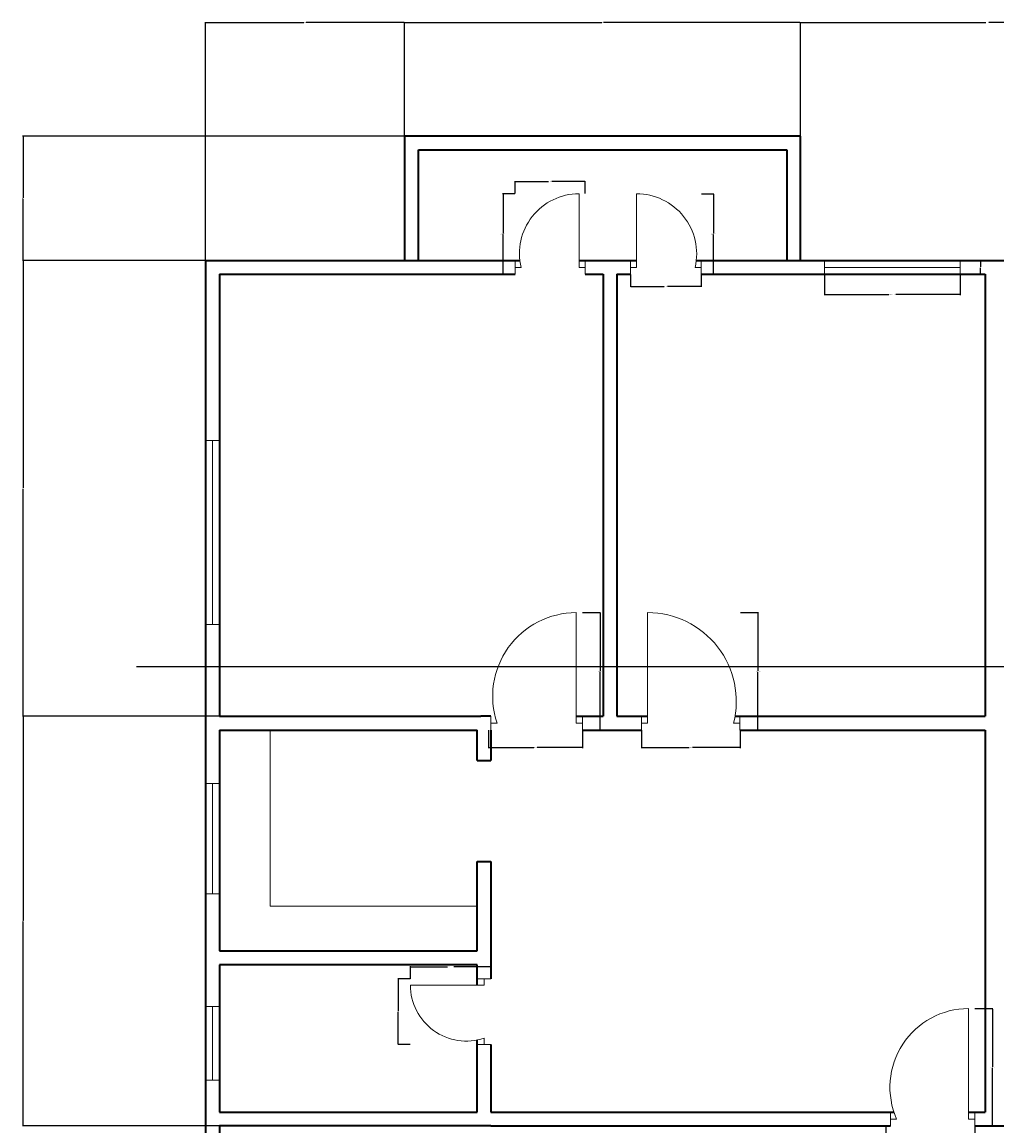
# Model space of a CAD drawing. Units: inches. Extents: x 1944 to 3454, y 1352 to 3055.
# Tile 13 of 17: x 2585 to 2903, y 1900 to 2260. Entities that reach past the tile are written whole.
import ezdxf

# ---------------------------------------------------------------- set-up
doc = ezdxf.new("R2010")
doc.units = ezdxf.units.IN
for name, color, linetype, lineweight in [('A-ANNO-DIMS', 2, 'Continuous', 18), ('A-ANNO-SYMB', 7, 'Continuous', 25), ('A-DOOR', 3, 'Continuous', 20), ('A-FLOR-CASE', 8, 'Continuous', 20), ('A-GLAZ', 4, 'Continuous', 18), ('A-WALL', 7, 'Continuous', 35)]:
    doc.layers.add(name, color=color, linetype=linetype, lineweight=lineweight)
doc.styles.get("Standard").update_dxf_attribs({"font": 'arial.ttf'})
doc.dimstyles.get("Standard").update_dxf_attribs({"dimtxt": 0.18, "dimasz": 0.18, "dimexe": 0.18, "dimexo": 0.0625, "dimgap": 0.09, "dimtad": 0, "dimtih": 1, "dimtoh": 1, "dimdec": 4, "dimzin": 0, "dimdsep": 46, "dimtxsty": 'Standard', "dimcen": 0.09, "dimadec": 0, "dimazin": 0, "dimtfac": 1, "dimtdec": 4, "dimtofl": 0, "dimtmove": 0, "dimatfit": 3, "dimfxl": 1, "dimtolj": 1, "dimtzin": 0, "dimarcsym": 0})

# ---------------------------------------------------------------- blocks, each defined once
blk = doc.blocks.new('DOOR-SWING-36IN-03')
for p, q in [((2, 2.25), (2, 38.25)), ((0, 4.5), (0, 0)), ((32, 4.5), (32, 0)), ((0, 0), (0, 2.25)), ((0, 2.25), (2, 2.25)), ((32, 2.25), (30, 2.25)), ((32, 0), (32, 2.25))]:
    blk.add_line(p, q)
blk.add_arc((2, 9.36), 28.89, 345.7565, 90)
blk = doc.blocks.new('DOOR-SWING-36IN-04')
for p, q in [((27.8, 2.25), (27.8, 38.25)), ((0, 0), (0, 4.5)), ((29.8, 4.5), (29.8, 0)), ((0, 2.25), (2, 2.25)), ((29.8, 2.25), (27.8, 2.25)), ((29.8, 0), (29.8, 2.25))]:
    blk.add_line(p, q)
blk.add_arc((27.8, 11), 27.25, 90, 198.7358)
blk = doc.blocks.new('DOOR-SWING-24IN-01')
for p, q in [((20.84, 2.25), (20.84, 26.25)), ((0, 4.5), (0, 0)), ((22.84, 0), (22.84, 4.5)), ((22.84, 4.5), (22.84, 2.25)), ((0, 0), (0, 2.25)), ((0, 2.25), (2, 2.25)), ((22.84, 2.25), (20.84, 2.25))]:
    blk.add_line(p, q)
blk.add_arc((20.84, 6.85), 19.4, 90, 193.7219)
blk = doc.blocks.new('DOOR-SWING-24IN-02')
for p, q in [((2, 2.25), (2, 26.25)), ((0, 0), (0, 4.5)), ((0, 4.5), (0, 2.25)), ((23.1, 4.5), (23.1, 0)), ((0, 2.25), (2, 2.25)), ((23.1, 2.25), (21.1, 2.25)), ((23.1, 0), (23.1, 2.25))]:
    blk.add_line(p, q)
blk.add_arc((2, 6.65), 19.6, 347.0256, 90)
blk = doc.blocks.new('DOOR-SWING-24IN-06')
for p, q in [((24, 19.31), (0, 19.31)), ((21.75, 21.31), (26.25, 21.31)), ((26.25, 21.31), (24, 21.31)), ((24, 21.31), (24, 19.31)), ((24, 0), (24, 2)), ((21.75, 0), (26.25, 0)), ((26.25, 0), (24, 0))]:
    blk.add_line(p, q)
blk.add_arc((18.24, 19.31), 18.24, 180, 288.4122)
blk = doc.blocks.new('DOOR-SWING-36IN-10')
for p, q in [((25.63, 2.25), (25.63, 38.25)), ((0.18, 4.5), (0.18, 0)), ((27.63, 4.5), (27.63, 0)), ((0.18, 0), (0.18, 2.25)), ((0.18, 2.25), (2.18, 2.25)), ((27.63, 2.25), (25.63, 2.25)), ((27.63, 0), (27.63, 2.25))]:
    blk.add_line(p, q)
blk.add_arc((25.63, 12.61), 25.64, 90, 203.8432)
blk = doc.blocks.new('WINDOW-PLAN-60.00IN-01')
for p, q in [((0, 60), (4.5, 60)), ((4.5, 60), (2.25, 60)), ((2.25, 60), (2.25, 0)), ((4.5, 0), (0, 0)), ((2.25, 0), (4.5, 0))]:
    blk.add_line(p, q)
blk = doc.blocks.new('WINDOW-PLAN-36.00IN-01')
for p, q in [((0, 36), (4.5, 36)), ((4.5, 36), (2.25, 36)), ((2.25, 36), (2.25, 0)), ((2.25, 0), (0, 0)), ((0, 0), (4.5, 0))]:
    blk.add_line(p, q)
blk = doc.blocks.new('WINDOW-PLAN-24.00IN-01')
for p, q in [((2.25, 24), (0, 24)), ((0, 24), (4.5, 24)), ((2.25, 0), (2.25, 24)), ((0, 0), (4.5, 0)), ((4.5, 0), (2.25, 0))]:
    blk.add_line(p, q)
blk = doc.blocks.new('WINDOW-PLAN-44.19IN-01')
for p, q in [((0, 4.5), (0, 0)), ((44.19, 2.25), (44.19, 4.5)), ((44.19, 4.5), (44.19, 0)), ((0, 0), (0, 2.25)), ((0, 2.25), (44.19, 2.25))]:
    blk.add_line(p, q)
blk = doc.blocks.new('*D86')
at = {"layer": 'A-ANNO-DIMS', "color": 0, "lineweight": -2, "transparency": 16777216}
for p, q in [((2846.55, 2177.53), (2846.55, 2170.79)), ((2890.74, 2177.53), (2890.74, 2170.79)), ((2846.73, 2170.97), (2867.52, 2170.97)), ((2890.56, 2170.97), (2869.76, 2170.97))]:
    blk.add_line(p, q, dxfattribs=at)
at = {"layer": 'A-ANNO-DIMS', "color": 0, "transparency": 16777216}
for points in [[(2846.73, 2171), (2846.73, 2170.94), (2846.55, 2170.97)], [(2890.56, 2171), (2890.56, 2170.94), (2890.74, 2170.97)]]:
    blk.add_solid(points, dxfattribs=at)
at = {"layer": 'Defpoints', "color": 0, "transparency": 16777216}
for p in [(2846.55, 2177.6), (2890.74, 2177.6), (2890.74, 2170.97)]:
    blk.add_point(p, dxfattribs=at)
at = {"layer": 'A-ANNO-DIMS', "color": 0, "transparency": 16777216, "insert": (2868.64, 2170.97), "char_height": 0.18, "attachment_point": 5}
blk.add_mtext('\\A1;WINDOW 44 TYP.', dxfattribs=at)
blk = doc.blocks.new('*D87')
at = {"layer": 'A-ANNO-DIMS', "color": 0, "lineweight": -2, "transparency": 16777216}
for p, q in [((2890.8, 2182.1), (2897.55, 2182.1)), ((2897.37, 2181.92), (2897.37, 2180.03)), ((2897.37, 2177.78), (2897.37, 2179.66)), ((2890.8, 2177.6), (2897.55, 2177.6))]:
    blk.add_line(p, q, dxfattribs=at)
at = {"layer": 'A-ANNO-DIMS', "color": 0, "transparency": 16777216}
for points in [[(2897.34, 2181.92), (2897.4, 2181.92), (2897.37, 2182.1)], [(2897.34, 2177.78), (2897.4, 2177.78), (2897.37, 2177.6)]]:
    blk.add_solid(points, dxfattribs=at)
at = {"layer": 'Defpoints', "color": 0, "transparency": 16777216}
for p in [(2890.74, 2182.1), (2897.37, 2182.1), (2890.74, 2177.6)]:
    blk.add_point(p, dxfattribs=at)
at = {"layer": 'A-ANNO-DIMS', "color": 0, "transparency": 16777216, "insert": (2897.37, 2179.85), "char_height": 0.18, "attachment_point": 5}
blk.add_mtext('\\A1;5 TYP.', dxfattribs=at)
blk = doc.blocks.new('*D96')
at = {"layer": 'A-ANNO-DIMS', "color": 0, "lineweight": -2, "transparency": 16777216}
for p, q in [((2819.16, 2067.35), (2825.02, 2067.35)), ((2824.84, 2067.17), (2824.84, 2048.4)), ((2824.84, 2029.28), (2824.84, 2048.04)), ((2819.16, 2029.1), (2825.02, 2029.1))]:
    blk.add_line(p, q, dxfattribs=at)
at = {"layer": 'A-ANNO-DIMS', "color": 0, "transparency": 16777216}
for points in [[(2824.81, 2067.17), (2824.87, 2067.17), (2824.84, 2067.35)], [(2824.81, 2029.28), (2824.87, 2029.28), (2824.84, 2029.1)]]:
    blk.add_solid(points, dxfattribs=at)
at = {"layer": 'Defpoints', "color": 0, "transparency": 16777216}
for p in [(2819.1, 2067.35), (2824.84, 2067.35), (2819.1, 2029.1)]:
    blk.add_point(p, dxfattribs=at)
at = {"layer": 'A-ANNO-DIMS', "color": 0, "transparency": 16777216, "insert": (2824.84, 2048.22), "char_height": 0.18, "attachment_point": 5}
blk.add_mtext('\\A1;SWING 38 TYP.', dxfattribs=at)
blk = doc.blocks.new('*D97')
at = {"layer": 'A-ANNO-DIMS', "color": 0, "lineweight": -2, "transparency": 16777216}
for p, q in [((2786.9, 2029.03), (2786.9, 2023.18)), ((2819.1, 2029.03), (2819.1, 2023.18)), ((2787.08, 2023.36), (2802.48, 2023.36)), ((2818.92, 2023.36), (2803.53, 2023.36))]:
    blk.add_line(p, q, dxfattribs=at)
at = {"layer": 'A-ANNO-DIMS', "color": 0, "transparency": 16777216}
for points in [[(2787.08, 2023.39), (2787.08, 2023.33), (2786.9, 2023.36)], [(2818.92, 2023.39), (2818.92, 2023.33), (2819.1, 2023.36)]]:
    blk.add_solid(points, dxfattribs=at)
at = {"layer": 'Defpoints', "color": 0, "transparency": 16777216}
for p in [(2786.9, 2029.1), (2819.1, 2029.1), (2819.1, 2023.36)]:
    blk.add_point(p, dxfattribs=at)
at = {"layer": 'A-ANNO-DIMS', "color": 0, "transparency": 16777216, "insert": (2803, 2023.36), "char_height": 0.18, "attachment_point": 5}
blk.add_mtext('\\A1;32 TYP.', dxfattribs=at)
blk = doc.blocks.new('*D98')
at = {"layer": 'A-ANNO-DIMS', "color": 0, "lineweight": -2, "transparency": 16777216}
for p, q in [((2767.74, 2067.35), (2773.6, 2067.35)), ((2773.42, 2067.17), (2773.42, 2048.4)), ((2773.42, 2029.28), (2773.42, 2048.04)), ((2767.74, 2029.1), (2773.6, 2029.1))]:
    blk.add_line(p, q, dxfattribs=at)
at = {"layer": 'A-ANNO-DIMS', "color": 0, "transparency": 16777216}
for points in [[(2773.39, 2067.17), (2773.45, 2067.17), (2773.42, 2067.35)], [(2773.39, 2029.28), (2773.45, 2029.28), (2773.42, 2029.1)]]:
    blk.add_solid(points, dxfattribs=at)
at = {"layer": 'Defpoints', "color": 0, "transparency": 16777216}
for p in [(2767.68, 2067.35), (2773.42, 2067.35), (2767.68, 2029.1)]:
    blk.add_point(p, dxfattribs=at)
at = {"layer": 'A-ANNO-DIMS', "color": 0, "transparency": 16777216, "insert": (2773.42, 2048.22), "char_height": 0.18, "attachment_point": 5}
blk.add_mtext('\\A1;SWING 38 TYP.', dxfattribs=at)
blk = doc.blocks.new('*D99')
at = {"layer": 'A-ANNO-DIMS', "color": 0, "lineweight": -2, "transparency": 16777216}
for p, q in [((2737.05, 2029.03), (2737.05, 2023.18)), ((2767.68, 2029.03), (2767.68, 2023.18)), ((2737.23, 2023.36), (2751.84, 2023.36)), ((2767.5, 2023.36), (2752.89, 2023.36))]:
    blk.add_line(p, q, dxfattribs=at)
at = {"layer": 'A-ANNO-DIMS', "color": 0, "transparency": 16777216}
for points in [[(2737.23, 2023.39), (2737.23, 2023.33), (2737.05, 2023.36)], [(2767.5, 2023.39), (2767.5, 2023.33), (2767.68, 2023.36)]]:
    blk.add_solid(points, dxfattribs=at)
at = {"layer": 'Defpoints', "color": 0, "transparency": 16777216}
for p in [(2737.05, 2029.1), (2767.68, 2029.1), (2767.68, 2023.36)]:
    blk.add_point(p, dxfattribs=at)
at = {"layer": 'A-ANNO-DIMS', "color": 0, "transparency": 16777216, "insert": (2752.37, 2023.36), "char_height": 0.18, "attachment_point": 5}
blk.add_mtext('\\A1;31 TYP.', dxfattribs=at)
blk = doc.blocks.new('*D110')
at = {"layer": 'A-ANNO-DIMS', "color": 0, "lineweight": -2, "transparency": 16777216}
for p, q in [((2895.56, 1938.35), (2901.41, 1938.35)), ((2901.23, 1938.17), (2901.23, 1919.4)), ((2901.23, 1900.28), (2901.23, 1919.04)), ((2895.56, 1900.1), (2901.41, 1900.1))]:
    blk.add_line(p, q, dxfattribs=at)
at = {"layer": 'A-ANNO-DIMS', "color": 0, "transparency": 16777216}
for points in [[(2901.2, 1938.17), (2901.26, 1938.17), (2901.23, 1938.35)], [(2901.2, 1900.28), (2901.26, 1900.28), (2901.23, 1900.1)]]:
    blk.add_solid(points, dxfattribs=at)
at = {"layer": 'Defpoints', "color": 0, "transparency": 16777216}
for p in [(2895.49, 1938.35), (2901.23, 1938.35), (2895.49, 1900.1)]:
    blk.add_point(p, dxfattribs=at)
at = {"layer": 'A-ANNO-DIMS', "color": 0, "transparency": 16777216, "insert": (2901.23, 1919.22), "char_height": 0.18, "attachment_point": 5}
blk.add_mtext('\\A1;SWING 38 TYP.', dxfattribs=at)
blk = doc.blocks.new('*D111')
at = {"layer": 'A-ANNO-DIMS', "color": 0, "lineweight": -2, "transparency": 16777216}
for p, q in [((2866.54, 1900.03), (2866.54, 1894.18)), ((2895.49, 1900.03), (2895.49, 1894.18)), ((2866.72, 1894.36), (2880.49, 1894.36)), ((2895.31, 1894.36), (2881.55, 1894.36))]:
    blk.add_line(p, q, dxfattribs=at)
at = {"layer": 'A-ANNO-DIMS', "color": 0, "transparency": 16777216}
for points in [[(2866.72, 1894.39), (2866.72, 1894.33), (2866.54, 1894.36)], [(2895.31, 1894.39), (2895.31, 1894.33), (2895.49, 1894.36)]]:
    blk.add_solid(points, dxfattribs=at)
at = {"layer": 'Defpoints', "color": 0, "transparency": 16777216}
for p in [(2866.54, 1900.1), (2895.49, 1900.1), (2895.49, 1894.36)]:
    blk.add_point(p, dxfattribs=at)
at = {"layer": 'A-ANNO-DIMS', "color": 0, "transparency": 16777216, "insert": (2881.02, 1894.36), "char_height": 0.18, "attachment_point": 5}
blk.add_mtext('\\A1;29 TYP.', dxfattribs=at)
blk = doc.blocks.new('*D116')
at = {"layer": 'A-ANNO-DIMS', "color": 0, "lineweight": -2, "transparency": 16777216}
for p, q in [((2745.67, 2203.85), (2741.62, 2203.85)), ((2741.8, 2203.67), (2741.8, 2190.9)), ((2741.8, 2177.78), (2741.8, 2190.54)), ((2745.67, 2177.6), (2741.62, 2177.6))]:
    blk.add_line(p, q, dxfattribs=at)
at = {"layer": 'A-ANNO-DIMS', "color": 0, "transparency": 16777216}
for points in [[(2741.77, 2203.67), (2741.83, 2203.67), (2741.8, 2203.85)], [(2741.77, 2177.78), (2741.83, 2177.78), (2741.8, 2177.6)]]:
    blk.add_solid(points, dxfattribs=at)
at = {"layer": 'Defpoints', "color": 0, "transparency": 16777216}
for p in [(2741.8, 2203.85), (2745.73, 2203.85), (2745.73, 2177.6)]:
    blk.add_point(p, dxfattribs=at)
at = {"layer": 'A-ANNO-DIMS', "color": 0, "transparency": 16777216, "insert": (2741.8, 2190.72), "char_height": 0.18, "attachment_point": 5}
blk.add_mtext('\\A1;SWING 26 TYP.', dxfattribs=at)
blk = doc.blocks.new('*D117')
at = {"layer": 'A-ANNO-DIMS', "color": 0, "lineweight": -2, "transparency": 16777216}
for p, q in [((2745.73, 2203.91), (2745.73, 2207.96)), ((2745.91, 2207.78), (2756.63, 2207.78)), ((2768.4, 2207.78), (2757.69, 2207.78)), ((2768.58, 2203.91), (2768.58, 2207.96))]:
    blk.add_line(p, q, dxfattribs=at)
at = {"layer": 'A-ANNO-DIMS', "color": 0, "transparency": 16777216}
for points in [[(2745.91, 2207.81), (2745.91, 2207.75), (2745.73, 2207.78)], [(2768.4, 2207.81), (2768.4, 2207.75), (2768.58, 2207.78)]]:
    blk.add_solid(points, dxfattribs=at)
at = {"layer": 'Defpoints', "color": 0, "transparency": 16777216}
for p in [(2768.58, 2207.78), (2745.73, 2203.85), (2768.58, 2203.85)]:
    blk.add_point(p, dxfattribs=at)
at = {"layer": 'A-ANNO-DIMS', "color": 0, "transparency": 16777216, "insert": (2757.16, 2207.78), "char_height": 0.18, "attachment_point": 5}
blk.add_mtext('\\A1;23 TYP.', dxfattribs=at)
blk = doc.blocks.new('*D118')
at = {"layer": 'A-ANNO-DIMS', "color": 0, "lineweight": -2, "transparency": 16777216}
for p, q in [((2806.45, 2203.85), (2810.51, 2203.85)), ((2810.33, 2203.67), (2810.33, 2190.9)), ((2810.33, 2177.78), (2810.33, 2190.54)), ((2806.45, 2177.6), (2810.51, 2177.6))]:
    blk.add_line(p, q, dxfattribs=at)
at = {"layer": 'A-ANNO-DIMS', "color": 0, "transparency": 16777216}
for points in [[(2810.3, 2203.67), (2810.36, 2203.67), (2810.33, 2203.85)], [(2810.3, 2177.78), (2810.36, 2177.78), (2810.33, 2177.6)]]:
    blk.add_solid(points, dxfattribs=at)
at = {"layer": 'Defpoints', "color": 0, "transparency": 16777216}
for p in [(2806.39, 2203.85), (2810.33, 2203.85), (2806.39, 2177.6)]:
    blk.add_point(p, dxfattribs=at)
at = {"layer": 'A-ANNO-DIMS', "color": 0, "transparency": 16777216, "insert": (2810.33, 2190.72), "char_height": 0.18, "attachment_point": 5}
blk.add_mtext('\\A1;SWING 26 TYP.', dxfattribs=at)
blk = doc.blocks.new('*D119')
at = {"layer": 'A-ANNO-DIMS', "color": 0, "lineweight": -2, "transparency": 16777216}
for p, q in [((2783.29, 2177.53), (2783.29, 2173.48)), ((2806.39, 2177.53), (2806.39, 2173.48)), ((2783.47, 2173.66), (2794.31, 2173.66)), ((2806.21, 2173.66), (2795.37, 2173.66))]:
    blk.add_line(p, q, dxfattribs=at)
at = {"layer": 'A-ANNO-DIMS', "color": 0, "transparency": 16777216}
for points in [[(2783.47, 2173.69), (2783.47, 2173.63), (2783.29, 2173.66)], [(2806.21, 2173.69), (2806.21, 2173.63), (2806.39, 2173.66)]]:
    blk.add_solid(points, dxfattribs=at)
at = {"layer": 'Defpoints', "color": 0, "transparency": 16777216}
for p in [(2783.29, 2177.6), (2806.39, 2177.6), (2806.39, 2173.66)]:
    blk.add_point(p, dxfattribs=at)
at = {"layer": 'A-ANNO-DIMS', "color": 0, "transparency": 16777216, "insert": (2794.84, 2173.66), "char_height": 0.18, "attachment_point": 5}
blk.add_mtext('\\A1;23 TYP.', dxfattribs=at)
blk = doc.blocks.new('*D126')
at = {"layer": 'A-ANNO-DIMS', "color": 0, "lineweight": -2, "transparency": 16777216}
for p, q in [((2711.63, 1948.05), (2711.63, 1952.1)), ((2711.81, 1951.92), (2723.76, 1951.92)), ((2737.7, 1951.92), (2725.74, 1951.92)), ((2737.88, 1948.05), (2737.88, 1952.1))]:
    blk.add_line(p, q, dxfattribs=at)
at = {"layer": 'A-ANNO-DIMS', "color": 0, "transparency": 16777216}
for points in [[(2711.81, 1951.95), (2711.81, 1951.89), (2711.63, 1951.92)], [(2737.7, 1951.95), (2737.7, 1951.89), (2737.88, 1951.92)]]:
    blk.add_solid(points, dxfattribs=at)
at = {"layer": 'Defpoints', "color": 0, "transparency": 16777216}
for p in [(2737.88, 1951.92), (2711.63, 1947.99), (2737.88, 1947.99)]:
    blk.add_point(p, dxfattribs=at)
at = {"layer": 'A-ANNO-DIMS', "color": 0, "transparency": 16777216, "insert": (2724.75, 1951.92), "char_height": 0.18, "attachment_point": 5}
blk.add_mtext('\\A1;SWING 26 TYP.', dxfattribs=at)
blk = doc.blocks.new('*D127')
at = {"layer": 'A-ANNO-DIMS', "color": 0, "lineweight": -2, "transparency": 16777216}
for p, q in [((2711.56, 1947.99), (2707.51, 1947.99)), ((2707.69, 1947.81), (2707.69, 1937.51)), ((2707.69, 1926.86), (2707.69, 1937.15)), ((2711.56, 1926.68), (2707.51, 1926.68))]:
    blk.add_line(p, q, dxfattribs=at)
at = {"layer": 'A-ANNO-DIMS', "color": 0, "transparency": 16777216}
for points in [[(2707.66, 1947.81), (2707.72, 1947.81), (2707.69, 1947.99)], [(2707.66, 1926.86), (2707.72, 1926.86), (2707.69, 1926.68)]]:
    blk.add_solid(points, dxfattribs=at)
at = {"layer": 'Defpoints', "color": 0, "transparency": 16777216}
for p in [(2707.69, 1947.99), (2711.63, 1947.99), (2711.63, 1926.68)]:
    blk.add_point(p, dxfattribs=at)
at = {"layer": 'A-ANNO-DIMS', "color": 0, "transparency": 16777216, "insert": (2707.69, 1937.33), "char_height": 0.18, "attachment_point": 5}
blk.add_mtext('\\A1;21 TYP.', dxfattribs=at)
blk = doc.blocks.new('*D188')
at = {"layer": 'A-ANNO-DIMS', "color": 0, "lineweight": -2, "transparency": 16777216}
for p, q in [((2644.81, 2182.1), (2585.24, 2182.1)), ((2585.42, 2181.92), (2585.42, 2108.03)), ((2585.42, 2033.78), (2585.42, 2107.66)), ((2649.31, 2033.6), (2585.24, 2033.6))]:
    blk.add_line(p, q, dxfattribs=at)
at = {"layer": 'A-ANNO-DIMS', "color": 0, "transparency": 16777216}
for points in [[(2585.39, 2181.92), (2585.45, 2181.92), (2585.42, 2182.1)], [(2585.39, 2033.78), (2585.45, 2033.78), (2585.42, 2033.6)]]:
    blk.add_solid(points, dxfattribs=at)
at = {"layer": 'Defpoints', "color": 0, "transparency": 16777216}
for p in [(2644.88, 2182.1), (2585.42, 2033.6), (2649.38, 2033.6)]:
    blk.add_point(p, dxfattribs=at)
at = {"layer": 'A-ANNO-DIMS', "color": 0, "transparency": 16777216, "insert": (2585.42, 2107.85), "char_height": 0.18, "attachment_point": 5}
blk.add_mtext('\\A1;148.5', dxfattribs=at)
blk = doc.blocks.new('*D189')
at = {"layer": 'A-ANNO-DIMS', "color": 0, "lineweight": -2, "transparency": 16777216}
for p, q in [((2649.31, 2033.6), (2585.24, 2033.6)), ((2585.42, 2033.42), (2585.42, 1967.03)), ((2585.42, 1900.28), (2585.42, 1966.66)), ((2649.31, 1900.1), (2585.24, 1900.1))]:
    blk.add_line(p, q, dxfattribs=at)
at = {"layer": 'A-ANNO-DIMS', "color": 0, "transparency": 16777216}
for points in [[(2585.39, 2033.42), (2585.45, 2033.42), (2585.42, 2033.6)], [(2585.39, 1900.28), (2585.45, 1900.28), (2585.42, 1900.1)]]:
    blk.add_solid(points, dxfattribs=at)
at = {"layer": 'Defpoints', "color": 0, "transparency": 16777216}
for p in [(2649.38, 2033.6), (2585.42, 1900.1), (2649.38, 1900.1)]:
    blk.add_point(p, dxfattribs=at)
at = {"layer": 'A-ANNO-DIMS', "color": 0, "transparency": 16777216, "insert": (2585.42, 1966.85), "char_height": 0.18, "attachment_point": 5}
blk.add_mtext('\\A1;133.5', dxfattribs=at)
blk = doc.blocks.new('*D193')
at = {"layer": 'A-ANNO-DIMS', "color": 0, "lineweight": -2, "transparency": 16777216}
for p, q in [((2709.66, 2222.6), (2585.24, 2222.6)), ((2585.42, 2222.42), (2585.42, 2202.53)), ((2585.42, 2182.28), (2585.42, 2202.16)), ((2644.81, 2182.1), (2585.24, 2182.1))]:
    blk.add_line(p, q, dxfattribs=at)
at = {"layer": 'A-ANNO-DIMS', "color": 0, "transparency": 16777216}
for points in [[(2585.39, 2222.42), (2585.45, 2222.42), (2585.42, 2222.6)], [(2585.39, 2182.28), (2585.45, 2182.28), (2585.42, 2182.1)]]:
    blk.add_solid(points, dxfattribs=at)
at = {"layer": 'Defpoints', "color": 0, "transparency": 16777216}
for p in [(2585.42, 2222.6), (2709.72, 2222.6), (2644.88, 2182.1)]:
    blk.add_point(p, dxfattribs=at)
at = {"layer": 'A-ANNO-DIMS', "color": 0, "transparency": 16777216, "insert": (2585.42, 2202.35), "char_height": 0.18, "attachment_point": 5}
blk.add_mtext('\\A1;40.5', dxfattribs=at)
blk = doc.blocks.new('*D194')
at = {"layer": 'A-ANNO-DIMS', "color": 0, "lineweight": -2, "transparency": 16777216}
for p, q in [((2644.88, 2182.16), (2644.88, 2259.78)), ((2645.06, 2259.6), (2676.9, 2259.6)), ((2709.54, 2259.6), (2677.69, 2259.6)), ((2709.72, 2222.66), (2709.72, 2259.78))]:
    blk.add_line(p, q, dxfattribs=at)
at = {"layer": 'A-ANNO-DIMS', "color": 0, "transparency": 16777216}
for points in [[(2645.06, 2259.63), (2645.06, 2259.57), (2644.88, 2259.6)], [(2709.54, 2259.63), (2709.54, 2259.57), (2709.72, 2259.6)]]:
    blk.add_solid(points, dxfattribs=at)
at = {"layer": 'Defpoints', "color": 0, "transparency": 16777216}
for p in [(2709.72, 2259.6), (2709.72, 2222.6), (2644.88, 2182.1)]:
    blk.add_point(p, dxfattribs=at)
at = {"layer": 'A-ANNO-DIMS', "color": 0, "transparency": 16777216, "insert": (2677.3, 2259.6), "char_height": 0.18, "attachment_point": 5}
blk.add_mtext('\\A1;64.85', dxfattribs=at)
blk = doc.blocks.new('*D195')
at = {"layer": 'A-ANNO-DIMS', "color": 0, "lineweight": -2, "transparency": 16777216}
for p, q in [((2709.72, 2222.66), (2709.72, 2259.78)), ((2709.9, 2259.6), (2773.94, 2259.6)), ((2838.54, 2259.6), (2774.5, 2259.6)), ((2838.72, 2222.66), (2838.72, 2259.78))]:
    blk.add_line(p, q, dxfattribs=at)
at = {"layer": 'A-ANNO-DIMS', "color": 0, "transparency": 16777216}
for points in [[(2709.9, 2259.63), (2709.9, 2259.57), (2709.72, 2259.6)], [(2838.54, 2259.63), (2838.54, 2259.57), (2838.72, 2259.6)]]:
    blk.add_solid(points, dxfattribs=at)
at = {"layer": 'Defpoints', "color": 0, "transparency": 16777216}
for p in [(2838.72, 2259.6), (2709.72, 2222.6), (2838.72, 2222.6)]:
    blk.add_point(p, dxfattribs=at)
at = {"layer": 'A-ANNO-DIMS', "color": 0, "transparency": 16777216, "insert": (2774.22, 2259.6), "char_height": 0.18, "attachment_point": 5}
blk.add_mtext('\\A1;129', dxfattribs=at)
blk = doc.blocks.new('*D196')
at = {"layer": 'A-ANNO-DIMS', "color": 0, "lineweight": -2, "transparency": 16777216}
for p, q in [((2838.72, 2222.66), (2838.72, 2259.78)), ((2838.9, 2259.6), (2899.14, 2259.6)), ((2960.29, 2259.6), (2900.05, 2259.6)), ((2960.47, 2222.66), (2960.47, 2259.78))]:
    blk.add_line(p, q, dxfattribs=at)
at = {"layer": 'A-ANNO-DIMS', "color": 0, "transparency": 16777216}
for points in [[(2838.9, 2259.63), (2838.9, 2259.57), (2838.72, 2259.6)], [(2960.29, 2259.63), (2960.29, 2259.57), (2960.47, 2259.6)]]:
    blk.add_solid(points, dxfattribs=at)
at = {"layer": 'Defpoints', "color": 0, "transparency": 16777216}
for p in [(2960.47, 2259.6), (2838.72, 2222.6), (2960.47, 2222.6)]:
    blk.add_point(p, dxfattribs=at)
at = {"layer": 'A-ANNO-DIMS', "color": 0, "transparency": 16777216, "insert": (2899.6, 2259.6), "char_height": 0.18, "attachment_point": 5}
blk.add_mtext('\\A1;121.75', dxfattribs=at)

msp = doc.modelspace()

# ---------------------------------------------------------------- linework, layer by layer
at = {"layer": 'A-ANNO-SYMB'}
msp.add_line((2622.416, 2049.778), (3208.282, 2049.778), dxfattribs=at)
at = {"layer": 'A-FLOR-CASE'}
for p, q in [((2665.961, 1971.658), (2665.961, 2029.096)), ((2733.375, 1971.658), (2665.961, 1971.658))]:
    msp.add_line(p, q, dxfattribs=at)
at = {"layer": 'A-WALL'}
for p, q in [((2714.221, 2222.596), (2709.721, 2222.596)), ((2709.721, 2222.596), (2709.721, 2182.096)), ((2838.721, 2222.596), (2714.221, 2222.596)), ((2838.721, 2218.096), (2838.721, 2222.596)), ((2714.221, 2182.096), (2714.221, 2218.096)), ((2714.221, 2218.096), (2798.221, 2218.096)), ((2798.221, 2218.096), (2822.221, 2218.096)), ((2822.221, 2218.096), (2834.221, 2218.096)), ((2834.221, 2218.096), (2834.221, 2182.096)), ((2838.721, 2182.096), (2838.721, 2218.096)), ((2644.875, 2182.096), (2747.324, 2182.096)), ((2644.875, 2182.096), (2644.875, 1530.096)), ((2766.579, 2182.096), (2785.292, 2182.096)), ((2804.773, 2182.096), (2996.655, 2182.096)), ((2834.221, 2182.096), (2838.721, 2182.096)), ((2649.375, 2177.596), (2745.734, 2177.596)), ((2649.375, 2177.596), (2649.375, 2033.596)), ((2768.579, 2177.596), (2774.375, 2177.596)), ((2774.375, 2177.596), (2774.375, 2033.596)), ((2778.875, 2177.596), (2783.292, 2177.596)), ((2778.875, 2177.596), (2778.875, 2033.596)), ((2806.391, 2177.596), (2898.875, 2177.596)), ((2898.875, 2177.596), (2898.875, 2033.596)), ((2649.375, 2033.596), (2734.575, 2033.596)), ((2737.875, 2033.596), (2734.575, 2033.596)), ((2765.679, 2033.596), (2774.375, 2033.596)), ((2778.875, 2033.596), (2788.905, 2033.596)), ((2817.385, 2033.596), (2898.875, 2033.596)), ((2649.375, 2029.096), (2732.842, 2029.096)), ((2649.375, 2029.096), (2649.375, 1957.096)), ((2732.842, 2029.096), (2733.375, 2029.096)), ((2733.375, 2019.118), (2733.375, 2029.096)), ((2737.875, 2029.096), (2737.875, 2019.118)), ((2767.679, 2029.096), (2786.905, 2029.096)), ((2818.908, 2029.096), (2898.875, 2029.096)), ((2898.875, 2029.096), (2898.875, 1904.596)), ((2733.375, 2019.118), (2737.875, 2019.118)), ((2733.375, 1957.096), (2733.375, 1986.22)), ((2733.375, 1986.22), (2737.875, 1986.22)), ((2737.875, 1986.22), (2737.875, 1957.096)), ((2649.375, 1957.096), (2733.375, 1957.096)), ((2737.875, 1957.096), (2737.875, 1952.596)), ((2649.375, 1952.596), (2649.375, 1904.596)), ((2733.375, 1952.596), (2649.375, 1952.596)), ((2733.375, 1945.985), (2733.375, 1952.596)), ((2737.875, 1952.596), (2737.875, 1947.985)), ((2733.375, 1904.596), (2733.375, 1928.087)), ((2737.875, 1926.68), (2737.875, 1904.596)), ((2649.375, 1904.596), (2733.375, 1904.596)), ((2737.875, 1904.596), (2869.175, 1904.596)), ((2893.494, 1904.596), (2898.875, 1904.596)), ((2649.375, 1900.096), (2649.375, 1840.096)), ((2737.875, 1900.096), (2649.375, 1900.096)), ((2649.375, 1900.096), (2649.375, 1840.096)), ((2737.875, 1900.096), (2868.046, 1900.096)), ((2895.494, 1900.096), (2906.831, 1900.096))]:
    msp.add_line(p, q, dxfattribs=at)

# ---------------------------------------------------------------- block references
at = {"layer": 'A-DOOR'}
for name, p in [('DOOR-SWING-24IN-01', (2745.735, 2177.596)), ('DOOR-SWING-24IN-02', (2783.292, 2177.596)), ('DOOR-SWING-36IN-04', (2737.876, 2029.096)), ('DOOR-SWING-36IN-03', (2786.905, 2029.096)), ('DOOR-SWING-24IN-06', (2711.626, 1926.68)), ('DOOR-SWING-36IN-10', (2867.863, 1900.096))]:
    msp.add_blockref(name, p, dxfattribs=at)
at = {"layer": 'A-GLAZ'}
for name, p in [('WINDOW-PLAN-44.19IN-01', (2846.547, 2177.596)), ('WINDOW-PLAN-60.00IN-01', (2644.876, 2063.452)), ('WINDOW-PLAN-36.00IN-01', (2644.876, 1975.678)), ('WINDOW-PLAN-24.00IN-01', (2644.876, 1914.977))]:
    msp.add_blockref(name, p, dxfattribs=at)

# ---------------------------------------------------------------- dimensions: what is measured, and where the dimension line sits
at = {"layer": 'A-ANNO-DIMS'}
for base, p1, p2, override, picture, middle in [((2709.721, 2259.596), (2644.875, 2182.096), (2709.721, 2222.596), {"dimdec": 2, "dimlfac": 1, "dimrnd": 0, "dimzin": 0, "dimdsep": 46, "dimlunit": 2}, '*D194', (2677.298, 2259.596)), ((2838.721, 2259.596), (2709.721, 2222.596), (2838.721, 2222.596), {"dimdec": 0, "dimlfac": 1, "dimrnd": 0, "dimzin": 0, "dimdsep": 46, "dimlunit": 2}, '*D195', (2774.221, 2259.596)), ((2960.47, 2259.596), (2838.721, 2222.596), (2960.47, 2222.596), {"dimdec": 2, "dimlfac": 1, "dimrnd": 0, "dimzin": 0, "dimdsep": 46, "dimlunit": 2}, '*D196', (2899.596, 2259.596))]:
    dim = msp.add_linear_dim(base=base, p1=p1, p2=p2, dimstyle='Standard', override=override, dxfattribs=at)
    dim.commit()
    dim.dimension.update_dxf_attribs({"geometry": picture, "text_midpoint": middle})
for base, p1, p2, picture, middle in [((2585.416, 2222.596), (2644.875, 2182.096), (2709.721, 2222.596), '*D193', (2585.416, 2202.346)), ((2585.416, 2033.596), (2644.875, 2182.096), (2649.375, 2033.596), '*D188', (2585.416, 2107.846)), ((2585.416, 1900.096), (2649.375, 2033.596), (2649.375, 1900.096), '*D189', (2585.416, 1966.846))]:
    dim = msp.add_linear_dim(base=base, p1=p1, p2=p2, angle=90, dimstyle='Standard', override={"dimdec": 1, "dimlfac": 1, "dimrnd": 0, "dimzin": 0, "dimdsep": 46, "dimlunit": 2}, dxfattribs=at)
    dim.commit()
    dim.dimension.update_dxf_attribs({"geometry": picture, "text_midpoint": middle})
for base, p1, p2, text, picture, middle in [((2768.579, 2207.784), (2745.734, 2203.846), (2768.579, 2203.846), '<> TYP.', '*D117', (2757.157, 2207.784)), ((2806.391, 2173.659), (2783.292, 2177.596), (2806.391, 2177.596), '<> TYP.', '*D119', (2794.842, 2173.659)), ((2890.74, 2170.967), (2846.547, 2177.596), (2890.74, 2177.596), 'WINDOW <> TYP.', '*D86', (2868.643, 2170.967)), ((2767.679, 2023.359), (2737.054, 2029.096), (2767.679, 2029.096), '<> TYP.', '*D99', (2752.367, 2023.359)), ((2819.102, 2023.359), (2786.905, 2029.096), (2819.102, 2029.096), '<> TYP.', '*D97', (2803.003, 2023.359)), ((2737.875, 1951.923), (2711.625, 1947.985), (2737.875, 1947.985), 'SWING <> TYP.', '*D126', (2724.75, 1951.923)), ((2895.494, 1894.359), (2866.541, 1900.096), (2895.494, 1900.096), '<> TYP.', '*D111', (2881.018, 1894.359))]:
    dim = msp.add_linear_dim(base=base, p1=p1, p2=p2, text=text, dimstyle='Standard', override={"dimdec": 0, "dimlfac": 1, "dimrnd": 0, "dimzin": 0, "dimdsep": 46, "dimlunit": 2}, dxfattribs=at)
    dim.commit()
    dim.dimension.update_dxf_attribs({"geometry": picture, "text_midpoint": middle})
for base, p1, p2, text, picture, middle in [((2741.797, 2203.846), (2745.734, 2177.596), (2745.734, 2203.846), 'SWING <> TYP.', '*D116', (2741.797, 2190.721)), ((2810.329, 2203.846), (2806.391, 2177.596), (2806.391, 2203.846), 'SWING <> TYP.', '*D118', (2810.329, 2190.721)), ((2897.368709076, 2182.096365033), (2890.739748374, 2177.596365033), (2890.739748374, 2182.096365033), '<> TYP.', '*D87', (2897.368709076, 2179.846365033)), ((2773.417, 2067.346), (2767.679, 2029.096), (2767.679, 2067.346), 'SWING <> TYP.', '*D98', (2773.417, 2048.221)), ((2824.839, 2067.346), (2819.102, 2029.096), (2819.102, 2067.346), 'SWING <> TYP.', '*D96', (2824.839, 2048.221)), ((2707.688, 1947.985), (2711.625, 1926.68), (2711.625, 1947.985), '<> TYP.', '*D127', (2707.688, 1937.332)), ((2901.232, 1938.346), (2895.494, 1900.096), (2895.494, 1938.346), 'SWING <> TYP.', '*D110', (2901.232, 1919.221))]:
    dim = msp.add_linear_dim(base=base, p1=p1, p2=p2, angle=90, text=text, dimstyle='Standard', override={"dimdec": 0, "dimlfac": 1, "dimrnd": 0, "dimzin": 0, "dimdsep": 46, "dimlunit": 2}, dxfattribs=at)
    dim.commit()
    dim.dimension.update_dxf_attribs({"geometry": picture, "text_midpoint": middle})

doc.saveas('drawing.dxf')
